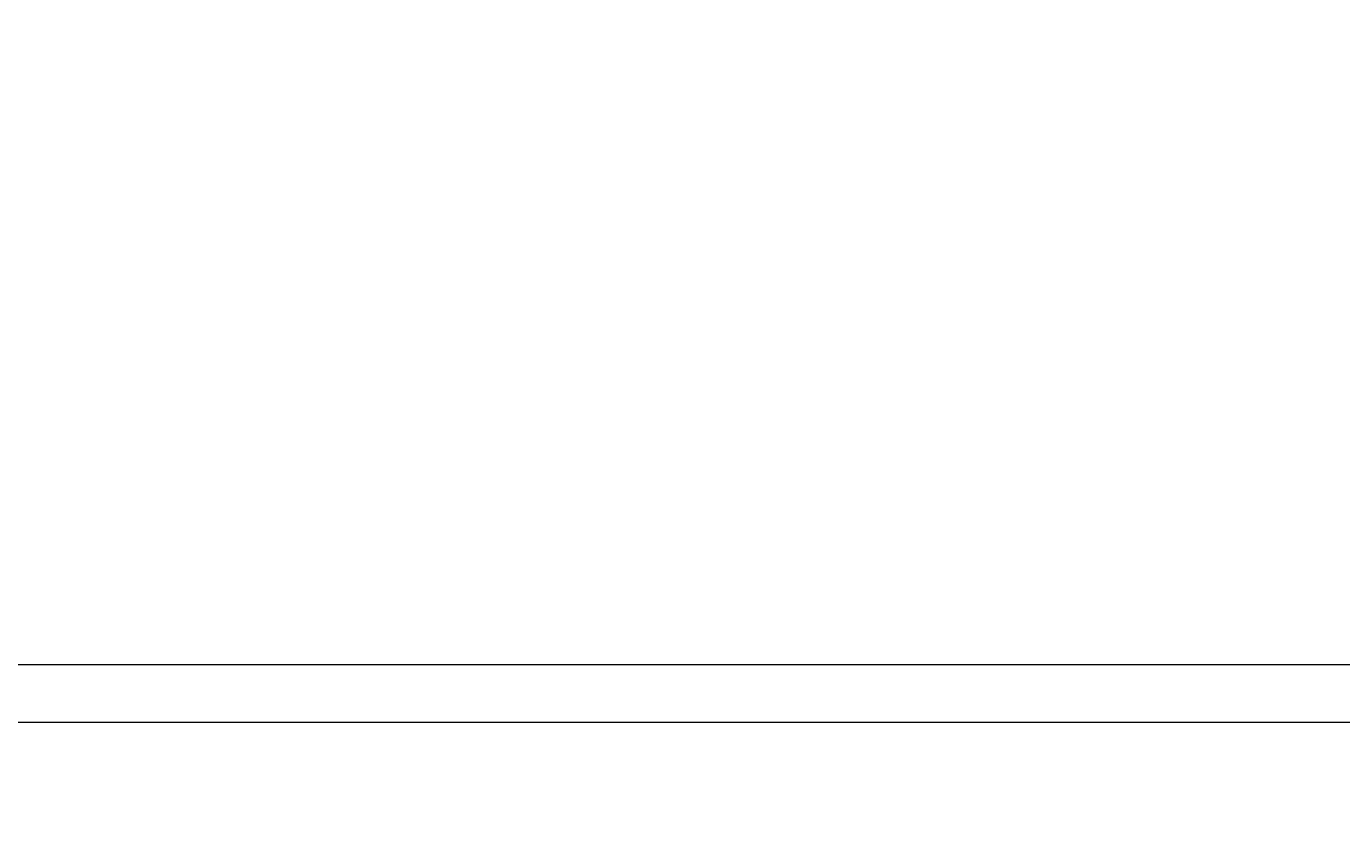
# Model space of a CAD drawing. Units: inches. Extents: x -61 to 1599, y -1316 to 257.
# Tile 118 of 204: x 134 to 161, y 11 to 27. Entities that reach past the tile are written whole.
import ezdxf

# ---------------------------------------------------------------- set-up
doc = ezdxf.new("R2010")
doc.units = ezdxf.units.IN
doc.header["$MEASUREMENT"] = 0
doc.layers.add('A-ANNO-DIMS', color=2, linetype='Continuous', lineweight=18)
doc.layers.add('FURNITURE', color=83, linetype='Continuous', lineweight=18)
doc.styles.get("Standard").update_dxf_attribs({"font": 'arial.ttf'})
doc.dimstyles.get("Standard").update_dxf_attribs({"dimtxt": 0.18, "dimasz": 0.18, "dimexe": 0.18, "dimexo": 0.0625, "dimgap": 0.09, "dimtad": 0, "dimtih": 1, "dimtoh": 1, "dimdec": 0, "dimzin": 0, "dimdsep": 46, "dimlunit": 3, "dimtxsty": 'Standard', "dimcen": 0.09, "dimadec": 0, "dimazin": 0, "dimtfac": 1, "dimtdec": 0, "dimtofl": 0, "dimtmove": 0, "dimatfit": 3, "dimfxl": 1, "dimtolj": 1, "dimtzin": 0, "dimarcsym": 0})

# ---------------------------------------------------------------- blocks, each defined once
blk = doc.blocks.new('BED-DOUBLE')
for p, q in [((1.272, 20.467), (70.263, 20.467)), ((1.272, 19.317), (70.263, 19.317))]:
    blk.add_line(p, q)
blk = doc.blocks.new('*D687')
at = {"layer": 'A-ANNO-DIMS', "color": 0, "lineweight": -2, "transparency": 16777216}
for p, q in [((289.418, 181.677), (-61.077, 181.677)), ((-60.897, 181.497), (-60.897, -528.952)), ((-60.897, -1239.765), (-60.897, -529.316)), ((319.64, -1239.945), (-61.077, -1239.945))]:
    blk.add_line(p, q, dxfattribs=at)
at = {"layer": 'A-ANNO-DIMS', "color": 0, "transparency": 16777216}
for points in [[(-60.927, 181.497), (-60.867, 181.497), (-60.897, 181.677)], [(-60.927, -1239.765), (-60.867, -1239.765), (-60.897, -1239.945)]]:
    blk.add_solid(points, dxfattribs=at)
at = {"layer": 'DEFPOINTS', "color": 0, "transparency": 16777216}
for p in [(289.481, 181.677), (-60.897, -1239.945), (319.703, -1239.945)]:
    blk.add_point(p, dxfattribs=at)
at = {"layer": 'A-ANNO-DIMS', "color": 0, "transparency": 16777216, "insert": (-60.897, -529.134), "char_height": 0.18, "attachment_point": 5}
blk.add_mtext('\\A1;1421.6', dxfattribs=at)
blk = doc.blocks.new('*D700')
at = {"layer": 'A-ANNO-DIMS', "color": 0, "lineweight": -2, "transparency": 16777216}
for p, q in [((14.703, -616.882), (14.703, 257.457)), ((179.752, -616.882), (179.752, 257.457)), ((14.883, 257.277), (96.772, 257.277)), ((179.572, 257.277), (97.683, 257.277))]:
    blk.add_line(p, q, dxfattribs=at)
at = {"layer": 'A-ANNO-DIMS', "color": 0, "transparency": 16777216}
for points in [[(14.883, 257.307), (14.883, 257.247), (14.703, 257.277)], [(179.572, 257.307), (179.572, 257.247), (179.752, 257.277)]]:
    blk.add_solid(points, dxfattribs=at)
at = {"layer": 'DEFPOINTS', "color": 0, "transparency": 16777216}
for p in [(179.752, 257.277), (14.703, -616.945), (179.752, -616.945)]:
    blk.add_point(p, dxfattribs=at)
at = {"layer": 'A-ANNO-DIMS', "color": 0, "transparency": 16777216, "insert": (97.227, 257.277), "char_height": 0.18, "attachment_point": 5}
blk.add_mtext('\\A1;165.05', dxfattribs=at)

msp = doc.modelspace()

# ---------------------------------------------------------------- block references
at = {"layer": 'FURNITURE'}
msp.add_blockref('BED-DOUBLE', (98.977, -5.797), dxfattribs=at)

# ---------------------------------------------------------------- dimensions: what is measured, and where the dimension line sits
at = {"layer": 'A-ANNO-DIMS'}
dim = msp.add_linear_dim(base=(179.7521, 257.2771), p1=(14.7028, -616.9446), p2=(179.7521, -616.9446), dimstyle='Standard', override={"dimdec": 2, "dimlfac": 1, "dimrnd": 0, "dimzin": 0, "dimdsep": 46, "dimlunit": 2}, dxfattribs=at)
dim.commit()
dim.dimension.update_dxf_attribs({"geometry": '*D700', "text_midpoint": (97.2274, 257.2771)})
dim = msp.add_linear_dim(base=(-60.8972, -1239.9446), p1=(289.4807, 181.6771), p2=(319.7028, -1239.9446), angle=90, dimstyle='Standard', override={"dimdec": 1, "dimlfac": 1, "dimrnd": 0, "dimzin": 0, "dimdsep": 46, "dimlunit": 2}, dxfattribs=at)
dim.commit()
dim.dimension.update_dxf_attribs({"geometry": '*D687', "text_midpoint": (-60.8972, -529.1337)})

doc.saveas('drawing.dxf')
